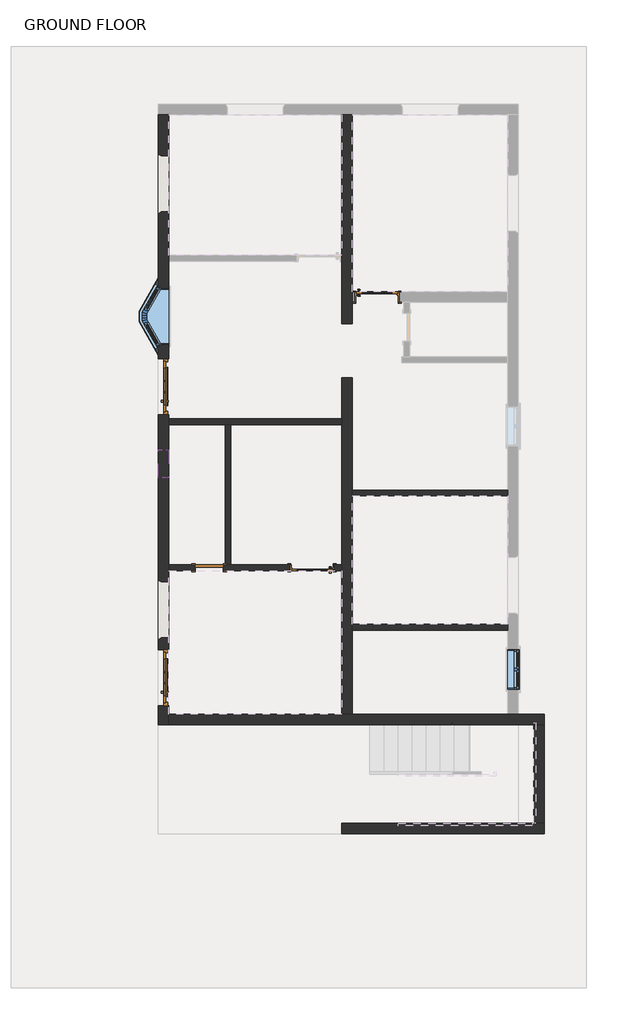
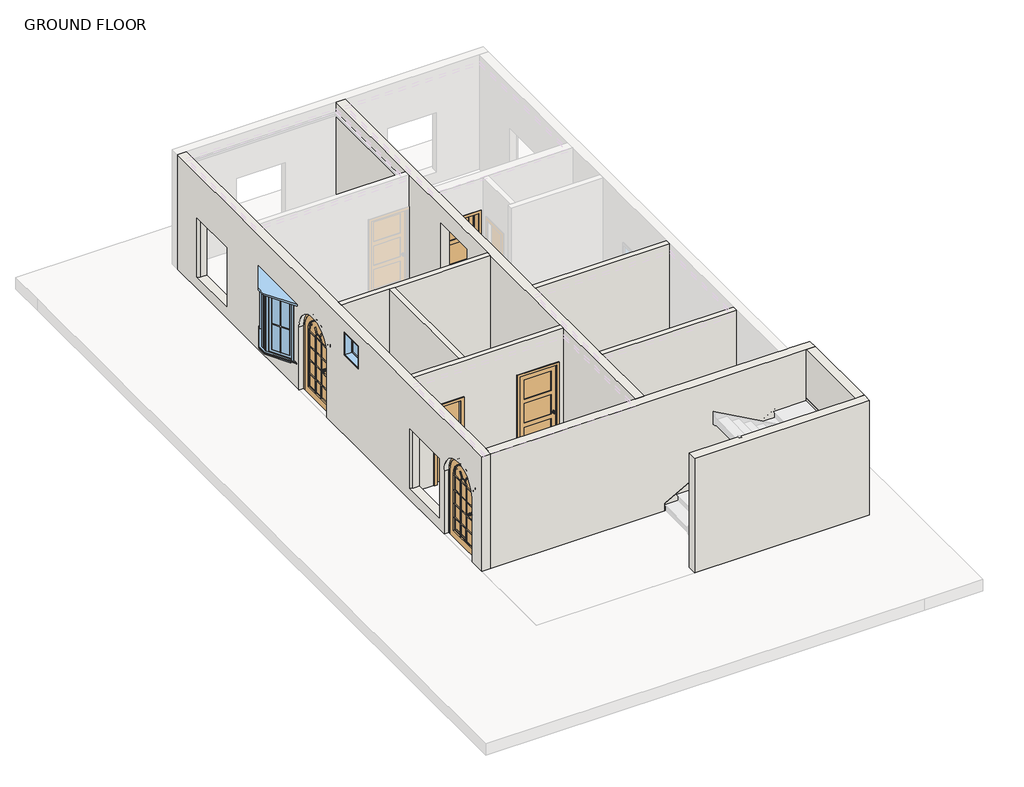
# One storey, part 1 of 2: 10 walls, 5 doors, 3 windows.
"""IFC4 building model written with IfcOpenShell, lengths in millimetres."""

from ifc_helpers import new_model, si_unit, frame, origin, place, context, project, spatial, polyline, circle_curve, outline, extrude, faceted_brep, transform, mapped, element, save
from ifc_brep_helpers import plane_surface, revolved_surface, advanced_brep
from components import door_interior_single_3_panel_vert_wood_interior_door_3_x_7_9905b5e2, door_interior_single_3_panel_vert_wood_interior_door_3_x_7_5540447a, door_arched_single_french_glass_wood_exterior_1219_x_2134mm_67be639c, single_flush_bathroom_flush_door_2_x_7_025d1c86, window_80340324, window_bay_casement_30_degree_angle_30_angle_window_doors_2_b97d1700, window_339605e1

model = new_model("IFC4")

# Units and contexts
model_context = context("Model", 3, world=origin())
ifc_project = project(units=[si_unit("LENGTHUNIT", "METRE", prefix="MILLI")], contexts=[model_context])

# Site, building, storey
site = spatial("IfcSite", under=ifc_project)
building = spatial("IfcBuilding", under=site)
storey = spatial("IfcBuildingStorey", under=building, Name="GROUND FLOOR", Elevation=304.8)

# Doors
placement = place(None, origin())
door_interior_single_3_panel_vert_wood_interior_door_3_x_7_shape = door_interior_single_3_panel_vert_wood_interior_door_3_x_7_9905b5e2(model_context)
element("IfcDoor", 1, ObjectType="Door-Interior-Single-3_Panel_Vert-Wood : 36\" x 84\"", at=placement, inside=storey, context=model_context, shape_type="MappedRepresentation", body=[
    mapped(door_interior_single_3_panel_vert_wood_interior_door_3_x_7_shape, transform((-12603.3436606, 7421.2725873, 304.8), x_axis=(1.0, 0.0, 0.0), y_axis=(0.0, 1.0, 0.0), z_axis=(0.0, 0.0, 1.0))),
])
door_interior_single_3_panel_vert_wood_interior_door_3_x_7_2_shape = door_interior_single_3_panel_vert_wood_interior_door_3_x_7_5540447a(model_context)
element("IfcDoor", 2, ObjectType="Door-Interior-Single-3_Panel_Vert-Wood : INTERIOR DOOR 3' X 7'", at=placement, inside=storey, context=model_context, shape_type="MappedRepresentation", body=[
    mapped(door_interior_single_3_panel_vert_wood_interior_door_3_x_7_2_shape, transform((-14013.0436606, 1534.8225873, 304.8), x_axis=(-1.0, 0.0, 0.0), y_axis=(0.0, -1.0, 0.0), z_axis=(0.0, 0.0, 1.0))),
])
door_arched_single_french_glass_wood_exterior_1219_x_2134mm_shape = door_arched_single_french_glass_wood_exterior_1219_x_2134mm_67be639c(model_context)
element("IfcDoor", 3, ObjectType="Door_Arched_Single_French_Glass_Wood_Exterior : 1219 x 2134mm", at=placement, inside=storey, context=model_context, shape_type="MappedRepresentation", body=[
    mapped(door_arched_single_french_glass_wood_exterior_1219_x_2134mm_shape, transform((-17238.8436606, -849.6024127, 304.8), x_axis=(0.0, 1.0, 0.0), y_axis=(-1.0, 0.0, 0.0), z_axis=(0.0, 0.0, 1.0))),
])
element("IfcDoor", 4, ObjectType="Door_Arched_Single_French_Glass_Wood_Exterior : 1219 x 2134mm", at=placement, inside=storey, context=model_context, shape_type="MappedRepresentation", body=[
    mapped(door_arched_single_french_glass_wood_exterior_1219_x_2134mm_shape, transform((-17238.8436606, 5474.9975873, 304.8), x_axis=(0.0, 1.0, 0.0), y_axis=(-1.0, 0.0, 0.0), z_axis=(0.0, 0.0, 1.0))),
])
single_flush_bathroom_flush_door_2_x_7_shape = single_flush_bathroom_flush_door_2_x_7_025d1c86(model_context)
element("IfcDoor", 5, ObjectType="Single-Flush : BATHROOM FLUSH DOOR 2' X 7'", at=placement, inside=storey, context=model_context, shape_type="MappedRepresentation", body=[
    mapped(single_flush_bathroom_flush_door_2_x_7_shape, transform((-16248.2436606, 1537.9975873, 304.8), x_axis=(1.0, 0.0, 0.0), y_axis=(0.0, 1.0, 0.0), z_axis=(0.0, 0.0, 1.0))),
])

# Walls
element("IfcWall", 6, at=placement, inside=storey, context=model_context, shape_type="AdvancedBrep", body=[
    advanced_brep(
    [(-17353.1436606, -1878.3024127, 3352.8), (-17353.1436606, 11380.4975873, 3352.8), (-17353.1436606, 11380.4975873, 304.8), (-17353.1436606, 6084.5975873, 304.8), (-17353.1436606, 6084.5975873, 1983.4), (-17353.1436606, 4865.3975873, 1983.4), (-17353.1436606, 4865.3975873, 304.8), (-17353.1436606, -240.0024127, 304.8), (-17353.1436606, -240.0024127, 1983.4), (-17353.1436606, -1459.2024127, 1983.4), (-17353.1436606, -1459.2024127, 304.8), (-17353.1436606, -1878.3024127, 304.8), (-17353.1436606, 1268.1225873, 2184.4), (-17353.1436606, -20.9274127, 2184.4), (-17353.1436606, -20.9274127, 609.6), (-17353.1436606, 1268.1225873, 609.6), (-17353.1436606, 3493.7975873, 3048.0), (-17353.1436606, 3493.7975873, 2438.4), (-17353.1436606, 4103.3975873, 2438.4), (-17353.1436606, 4103.3975873, 3048.0), (-17353.1436606, 7643.5225873, 2489.2), (-17353.1436606, 6354.4725873, 2489.2), (-17353.1436606, 6354.4725873, 914.4), (-17353.1436606, 7643.5225873, 914.4), (-17353.1436606, 10526.4225873, 2184.4), (-17353.1436606, 9237.3725873, 2184.4), (-17353.1436606, 9237.3725873, 609.6), (-17353.1436606, 10526.4225873, 609.6), (-17124.5436606, 11380.4975873, 3352.8), (-17124.5436606, 8332.4975873, 3352.8), (-17124.5436606, 8205.4975873, 3352.8), (-17124.5436606, 4776.4975873, 3352.8), (-17124.5436606, 4649.4975873, 3352.8), (-17124.5436606, 1601.4975873, 3352.8), (-17124.5436606, 1474.4975873, 3352.8), (-17124.5436606, -1649.7024127, 3352.8), (-17124.5436606, -1878.3024127, 3352.8), (-17124.5436606, -1878.3024127, 304.8), (-17124.5436606, -1649.7024127, 304.8), (-17124.5436606, -1459.2024127, 304.8), (-17124.5436606, -1459.2024127, 1983.4), (-17124.5436606, -240.0024127, 1983.4), (-17124.5436606, -240.0024127, 304.8), (-17124.5436606, 1474.4975873, 304.8), (-17124.5436606, 1601.4975873, 304.8), (-17124.5436606, 4649.4975873, 304.8), (-17124.5436606, 4776.4975873, 304.8), (-17124.5436606, 4865.3975873, 304.8), (-17124.5436606, 4865.3975873, 1983.4), (-17124.5436606, 6084.5975873, 1983.4), (-17124.5436606, 6084.5975873, 304.8), (-17124.5436606, 8205.4975873, 304.8), (-17124.5436606, 8332.4975873, 304.8), (-17124.5436606, 11380.4975873, 304.8), (-17124.5436606, 13.9975873, 2184.4), (-17124.5436606, 1233.1975873, 2184.4), (-17124.5436606, 1233.1975873, 609.6), (-17124.5436606, 13.9975873, 609.6), (-17124.5436606, 3493.7975873, 2438.4), (-17124.5436606, 3493.7975873, 3048.0), (-17124.5436606, 4103.3975873, 3048.0), (-17124.5436606, 4103.3975873, 2438.4), (-17124.5436606, 6389.3975873, 2489.2), (-17124.5436606, 7608.5975873, 2489.2), (-17124.5436606, 7608.5975873, 914.4), (-17124.5436606, 6389.3975873, 914.4), (-17124.5436606, 9272.2975873, 2184.4), (-17124.5436606, 10491.4975873, 2184.4), (-17124.5436606, 10491.4975873, 609.6), (-17124.5436606, 9272.2975873, 609.6), (-17292.6517862, 13.9975873, 2184.4), (-17292.6517862, 1233.1975873, 2184.4), (-17292.6517862, 13.9975873, 609.6), (-17292.6517862, 1233.1975873, 609.6), (-17292.6517862, 6389.3975873, 2489.2), (-17292.6517862, 7608.5975873, 2489.2), (-17292.6517862, 6389.3975873, 914.4), (-17292.6517862, 7608.5975873, 914.4), (-17292.6517862, 9272.2975873, 2184.4), (-17292.6517862, 10491.4975873, 2184.4), (-17292.6517862, 9272.2975873, 609.6), (-17292.6517862, 10491.4975873, 609.6)],
    [
        (0, 1),
        (1, 2),
        (2, 3),
        (3, 4),
        (4, 5, circle_curve(frame((-17353.1436606, 5474.9975873, 1983.4), z_axis=(1.0, 0.0, 0.0), x_axis=(0.0, 1.0, 0.0)), 609.6)),
        (5, 6),
        (6, 7),
        (7, 8),
        (8, 9, circle_curve(frame((-17353.1436606, -849.6024127, 1983.4), z_axis=(1.0, 0.0, 0.0), x_axis=(0.0, 1.0, 0.0)), 609.6)),
        (9, 10),
        (10, 11),
        (11, 0),
        (12, 13),
        (13, 14),
        (14, 15),
        (15, 12),
        (16, 17),
        (17, 18),
        (18, 19),
        (19, 16),
        (20, 21),
        (21, 22),
        (22, 23),
        (23, 20),
        (24, 25),
        (25, 26),
        (26, 27),
        (27, 24),
        (28, 29),
        (29, 30),
        (30, 31),
        (31, 32),
        (32, 33),
        (33, 34),
        (34, 35),
        (35, 36),
        (36, 37),
        (37, 38),
        (38, 39),
        (39, 40),
        (40, 41, circle_curve(frame((-17124.5436606, -849.6024127, 1983.4), z_axis=(-1.0, 0.0, 0.0), x_axis=(0.0, 1.0, 0.0)), 609.6)),
        (41, 42),
        (42, 43),
        (43, 44),
        (44, 45),
        (45, 46),
        (46, 47),
        (47, 48),
        (48, 49, circle_curve(frame((-17124.5436606, 5474.9975873, 1983.4), z_axis=(-1.0, 0.0, 0.0), x_axis=(0.0, 1.0, 0.0)), 609.6)),
        (49, 50),
        (50, 51),
        (51, 52),
        (52, 53),
        (53, 28),
        (54, 55),
        (55, 56),
        (56, 57),
        (57, 54),
        (58, 59),
        (59, 60),
        (60, 61),
        (61, 58),
        (62, 63),
        (63, 64),
        (64, 65),
        (65, 62),
        (66, 67),
        (67, 68),
        (68, 69),
        (69, 66),
        (2, 53),
        (50, 3),
        (37, 11),
        (10, 39),
        (42, 7),
        (6, 47),
        (0, 36),
        (28, 1),
        (70, 13),
        (12, 71),
        (71, 55),
        (54, 70),
        (72, 57),
        (56, 73),
        (73, 15),
        (14, 72),
        (72, 70),
        (71, 73),
        (8, 41),
        (40, 9),
        (4, 49),
        (48, 5),
        (16, 59),
        (58, 17),
        (61, 18),
        (60, 19),
        (74, 21),
        (20, 75),
        (75, 63),
        (62, 74),
        (76, 65),
        (64, 77),
        (77, 23),
        (22, 76),
        (76, 74),
        (75, 77),
        (78, 25),
        (24, 79),
        (79, 67),
        (66, 78),
        (80, 69),
        (68, 81),
        (81, 27),
        (26, 80),
        (80, 78),
        (79, 81),
    ],
    [
        plane_surface(frame((-17353.1436606, 11380.4975873, 304.8), z_axis=(-1.0, 0.0, 0.0), x_axis=(0.0, -1.0, 0.0))),
        plane_surface(frame((-17124.5436606, 11380.4975873, 304.8), z_axis=(1.0, 0.0, 0.0), x_axis=(0.0, 1.0, 0.0))),
        plane_surface(frame((-17353.1436606, 11494.7975873, 304.8), z_axis=(0.0, 0.0, -1.0), x_axis=(1.0, 0.0, 0.0))),
        plane_surface(frame((-17353.1436606, -1764.0024127, 3352.8), z_axis=(0.0, 0.0, 1.0), x_axis=(1.0, 0.0, 0.0))),
        plane_surface(frame((-17325.7404762, 11380.4975873, 304.8), z_axis=(0.0, 1.0, 0.0), x_axis=(1.0, 0.0, 0.0))),
        plane_surface(frame((-17353.1436606, -1878.3024127, 304.8), z_axis=(0.0, -1.0, 0.0), x_axis=(1.0, 0.0, 0.0))),
        plane_surface(frame((-17292.6517862, 13.9975873, 2184.4), z_axis=(0.0, 0.0, -1.0), x_axis=(1.0, 0.0, 0.0))),
        plane_surface(frame((-17292.6517862, 13.9975873, 609.6), z_axis=(0.0, 0.0, 1.0), x_axis=(-1.0, 0.0, 0.0))),
        plane_surface(frame((-17292.6517862, 13.9975873, 2184.4), z_axis=(0.0, 1.0, 0.0), x_axis=(0.0, 0.0, -1.0))),
        plane_surface(frame((-17124.5436606, 1233.1975873, 2184.4), z_axis=(0.0, -1.0, 0.0), x_axis=(0.0, 0.0, -1.0))),
        plane_surface(frame((-17292.6517862, 1233.1975873, 2184.4), z_axis=(-0.5000000000000007, -0.8660254037844383, 0.0), x_axis=(0.0, 0.0, -1.0))),
        plane_surface(frame((-17353.1436606, -20.9274127, 2184.4), z_axis=(-0.4999999999999979, 0.8660254037844399, 0.0), x_axis=(0.0, 0.0, -1.0))),
        revolved_surface(polyline([(-17124.5436606, -240.00241269999992, 1983.4), (-17353.1436606, -240.00241269999992, 1983.4)]), (-17353.1436606, -849.6024127, 1983.4), (1.0, 0.0, 0.0)),
        plane_surface(frame((-17353.1436606, -1459.2024127, 1983.4), z_axis=(0.0, 1.0, 0.0), x_axis=(1.0, 0.0, 0.0))),
        plane_surface(frame((-17353.1436606, -240.0024127, 304.8), z_axis=(0.0, -1.0, 0.0), x_axis=(1.0, 0.0, 0.0))),
        revolved_surface(polyline([(-17124.5436606, 6084.597587300001, 1983.4), (-17353.1436606, 6084.597587300001, 1983.4)]), (-17353.1436606, 5474.9975873, 1983.4), (1.0, 0.0, 0.0)),
        plane_surface(frame((-17353.1436606, 4865.3975873, 1983.4), z_axis=(0.0, 1.0, 0.0), x_axis=(1.0, 0.0, 0.0))),
        plane_surface(frame((-17353.1436606, 6084.5975873, 304.8), z_axis=(0.0, -1.0, 0.0), x_axis=(1.0, 0.0, 0.0))),
        plane_surface(frame((-17353.1436606, 3493.7975873, 3048.0), z_axis=(0.0, 1.0, 0.0), x_axis=(1.0, 0.0, 0.0))),
        plane_surface(frame((-17353.1436606, 3493.7975873, 2438.4), z_axis=(0.0, 0.0, 1.0), x_axis=(1.0, 0.0, 0.0))),
        plane_surface(frame((-17353.1436606, 4103.3975873, 2438.4), z_axis=(0.0, -1.0, 0.0), x_axis=(1.0, 0.0, 0.0))),
        plane_surface(frame((-17353.1436606, 4103.3975873, 3048.0), z_axis=(0.0, 0.0, -1.0), x_axis=(1.0, 0.0, 0.0))),
        plane_surface(frame((-17292.6517862, 6389.3975873, 2489.2), z_axis=(0.0, 0.0, -1.0), x_axis=(1.0, 0.0, 0.0))),
        plane_surface(frame((-17292.6517862, 6389.3975873, 914.4), z_axis=(0.0, 0.0, 1.0), x_axis=(-1.0, 0.0, 0.0))),
        plane_surface(frame((-17292.6517862, 6389.3975873, 2489.2), z_axis=(0.0, 1.0, 0.0), x_axis=(0.0, 0.0, -1.0))),
        plane_surface(frame((-17124.5436606, 7608.5975873, 2489.2), z_axis=(0.0, -1.0, 0.0), x_axis=(0.0, 0.0, -1.0))),
        plane_surface(frame((-17292.6517862, 7608.5975873, 2489.2), z_axis=(-0.5000000000000007, -0.8660254037844383, 0.0), x_axis=(0.0, 0.0, -1.0))),
        plane_surface(frame((-17353.1436606, 6354.4725873, 2489.2), z_axis=(-0.4999999999999979, 0.8660254037844399, 0.0), x_axis=(0.0, 0.0, -1.0))),
        plane_surface(frame((-17292.6517862, 9272.2975873, 2184.4), z_axis=(0.0, 0.0, -1.0), x_axis=(1.0, 0.0, 0.0))),
        plane_surface(frame((-17292.6517862, 9272.2975873, 609.6), z_axis=(0.0, 0.0, 1.0), x_axis=(-1.0, 0.0, 0.0))),
        plane_surface(frame((-17292.6517862, 9272.2975873, 2184.4), z_axis=(0.0, 1.0, 0.0), x_axis=(0.0, 0.0, -1.0))),
        plane_surface(frame((-17124.5436606, 10491.4975873, 2184.4), z_axis=(0.0, -1.0, 0.0), x_axis=(0.0, 0.0, -1.0))),
        plane_surface(frame((-17292.6517862, 10491.4975873, 2184.4), z_axis=(-0.5000000000000007, -0.8660254037844383, 0.0), x_axis=(0.0, 0.0, -1.0))),
        plane_surface(frame((-17353.1436606, 9237.3725873, 2184.4), z_axis=(-0.4999999999999979, 0.8660254037844399, 0.0), x_axis=(0.0, 0.0, -1.0))),
    ],
    [
        (0, [[1, 2, 3, 4, 5, 6, 7, 8, 9, 10, 11, 12], [13, 14, 15, 16], [17, 18, 19, 20], [21, 22, 23, 24], [25, 26, 27, 28]]),
        (1, [[29, 30, 31, 32, 33, 34, 35, 36, 37, 38, 39, 40, 41, 42, 43, 44, 45, 46, 47, 48, 49, 50, 51, 52, 53, 54], [55, 56, 57, 58], [59, 60, 61, 62], [63, 64, 65, 66], [67, 68, 69, 70]]),
        (2, [[71, -53, -52, -51, 72, -3]]),
        (2, [[73, -11, 74, -39, -38]]),
        (2, [[75, -7, 76, -47, -46, -45, -44, -43]]),
        (3, [[-1, 77, -36, -35, -34, -33, -32, -31, -30, -29, 78]]),
        (4, [[-2, -78, -54, -71]]),
        (5, [[-12, -73, -37, -77]]),
        (6, [[79, -13, 80, 81, -55, 82]]),
        (7, [[83, -57, 84, 85, -15, 86]]),
        (8, [[-82, -58, -83, 87]]),
        (9, [[-81, 88, -84, -56]]),
        (10, [[-80, -16, -85, -88]]),
        (11, [[-79, -87, -86, -14]]),
        (12, [[-9, 89, -41, 90]]),
        (13, [[-10, -90, -40, -74]]),
        (14, [[-8, -75, -42, -89]]),
        (15, [[-5, 91, -49, 92]]),
        (16, [[-6, -92, -48, -76]]),
        (17, [[-4, -72, -50, -91]]),
        (18, [[-17, 93, -59, 94]]),
        (19, [[-18, -94, -62, 95]]),
        (20, [[-19, -95, -61, 96]]),
        (21, [[-20, -96, -60, -93]]),
        (22, [[97, -21, 98, 99, -63, 100]]),
        (23, [[101, -65, 102, 103, -23, 104]]),
        (24, [[-100, -66, -101, 105]]),
        (25, [[-99, 106, -102, -64]]),
        (26, [[-98, -24, -103, -106]]),
        (27, [[-97, -105, -104, -22]]),
        (28, [[107, -25, 108, 109, -67, 110]]),
        (29, [[111, -69, 112, 113, -27, 114]]),
        (30, [[-110, -70, -111, 115]]),
        (31, [[-109, 116, -112, -68]]),
        (32, [[-108, -28, -113, -116]]),
        (33, [[-107, -115, -114, -26]]),
    ],
),
])
element("IfcWall", 7, at=placement, inside=storey, context=model_context, shape_type="Brep", body=[
    faceted_brep([(-17124.5436606, -1878.3024127, 304.8), (-9199.7436606, -1878.3024127, 304.8), (-8971.1436606, -1878.3024127, 304.8), (-8971.1436606, -1878.3024127, 3352.8), (-9199.7436606, -1878.3024127, 3352.8), (-17124.5436606, -1878.3024127, 3352.8), (-17124.5436606, -1649.7024127, 304.8), (-17124.5436606, -1649.7024127, 3352.8), (-13365.3436606, -1649.7024127, 3352.8), (-13136.7436606, -1649.7024127, 3352.8), (-9758.5436606, -1649.7024127, 3352.8), (-9529.9436606, -1649.7024127, 3352.8), (-8971.1436606, -1649.7024127, 3352.8), (-8971.1436606, -1649.7024127, 304.8), (-9529.9436606, -1649.7024127, 304.8), (-9758.5436606, -1649.7024127, 304.8), (-13136.7436606, -1649.7024127, 304.8), (-13365.3436606, -1649.7024127, 304.8)], [[[0, 1, 2, 3, 4, 5]], [[6, 7, 8, 9, 10, 11, 12, 13, 14, 15, 16, 17]], [[2, 1, 0, 6, 17, 16, 15, 14, 13]], [[5, 4, 3, 12, 11, 10, 9, 8, 7]], [[0, 5, 7, 6]], [[3, 2, 13, 12]]]),
])
element("IfcWall", 8, at=placement, inside=storey, context=model_context, shape_type="Brep", body=[
    faceted_brep([(-13365.3436606, -1649.7024127, 304.8), (-13365.3436606, -1649.7024127, 3352.8), (-13365.3436606, 1474.4975873, 3352.8), (-13365.3436606, 1601.4975873, 3352.8), (-13365.3436606, 4649.4975873, 3352.8), (-13365.3436606, 4776.4975873, 3352.8), (-13365.3436606, 8205.4975873, 3352.8), (-13365.3436606, 8332.4975873, 3352.8), (-13365.3436606, 11380.4975873, 3352.8), (-13365.3436606, 11380.4975873, 304.8), (-13365.3436606, 8332.4975873, 304.8), (-13365.3436606, 8205.4975873, 304.8), (-13365.3436606, 6840.0734188, 304.8), (-13365.3436606, 6840.0734188, 2912.3433381), (-13365.3436606, 5663.8725029, 2912.3433381), (-13365.3436606, 5663.8725029, 304.8), (-13365.3436606, 4776.4975873, 304.8), (-13365.3436606, 4649.4975873, 304.8), (-13365.3436606, 1601.4975873, 304.8), (-13365.3436606, 1474.4975873, 304.8), (-13136.7436606, -1649.7024127, 3352.8), (-13136.7436606, -1649.7024127, 304.8), (-13136.7436606, 179.0975873, 304.8), (-13136.7436606, 306.0975873, 304.8), (-13136.7436606, 3100.0975873, 304.8), (-13136.7436606, 3227.0975873, 304.8), (-13136.7436606, 5663.8725029, 304.8), (-13136.7436606, 5663.8725029, 2912.3433381), (-13136.7436606, 6840.0734188, 2912.3433381), (-13136.7436606, 6840.0734188, 304.8), (-13136.7436606, 7303.7975873, 304.8), (-13136.7436606, 7532.3975873, 304.8), (-13136.7436606, 11380.4975873, 304.8), (-13136.7436606, 11380.4975873, 3352.8), (-13136.7436606, 7532.3975873, 3352.8), (-13136.7436606, 7303.7975873, 3352.8), (-13136.7436606, 3227.0975873, 3352.8), (-13136.7436606, 3100.0975873, 3352.8), (-13136.7436606, 306.0975873, 3352.8), (-13136.7436606, 179.0975873, 3352.8)], [[[0, 1, 2, 3, 4, 5, 6, 7, 8, 9, 10, 11, 12, 13, 14, 15, 16, 17, 18, 19]], [[20, 21, 22, 23, 24, 25, 26, 27, 28, 29, 30, 31, 32, 33, 34, 35, 36, 37, 38, 39]], [[9, 8, 33, 32]], [[1, 0, 21, 20]], [[13, 28, 27, 14]], [[28, 13, 12, 29]], [[14, 27, 26, 15]], [[9, 32, 31, 30, 29, 12, 11, 10]], [[21, 0, 19, 18, 17, 16, 15, 26, 25, 24, 23, 22]], [[8, 7, 6, 5, 4, 3, 2, 1, 20, 39, 38, 37, 36, 35, 34, 33]]]),
])
element("IfcWall", 9, at=placement, inside=storey, context=model_context, shape_type="Brep", body=[
    faceted_brep([(-13365.3436606, -4240.5024127, 304.8), (-8971.1436606, -4240.5024127, 304.8), (-8971.1436606, -4240.5024127, 3352.8), (-13365.3436606, -4240.5024127, 3352.8), (-13365.3436606, -4011.9024127, 304.8), (-13365.3436606, -4011.9024127, 3352.8), (-9199.7436606, -4011.9024127, 3352.8), (-8971.1436606, -4011.9024127, 3352.8), (-8971.1436606, -4011.9024127, 304.8), (-9199.7436606, -4011.9024127, 304.8)], [[[0, 1, 2, 3]], [[4, 5, 6, 7, 8, 9]], [[1, 0, 4, 9, 8]], [[3, 2, 7, 6, 5]], [[0, 3, 5, 4]], [[2, 1, 8, 7]]]),
])
element("IfcWall", 10, at=placement, inside=storey, context=model_context, shape_type="SweptSolid", body=[
    extrude(outline(polyline([(-8971.1436606, -1878.3024127), (-8971.1436606, -4011.9024127), (-9199.7436606, -4011.9024127), (-9199.7436606, -1878.3024127), (-8971.1436606, -1878.3024127)])), frame((0.0, 0.0, 304.8), z_axis=(0.0, 0.0, 1.0), x_axis=(1.0, 0.0, 0.0)), (0.0, 0.0, 1.0), 3048.0),
])
element("IfcWall", 11, ObjectType="INNER WALL 5\"", at=placement, inside=storey, context=model_context, shape_type="Brep", body=[
    faceted_brep([(-17124.5436606, 4649.4975873, 304.8), (-15905.3436606, 4649.4975873, 304.8), (-15778.3436606, 4649.4975873, 304.8), (-13365.3436606, 4649.4975873, 304.8), (-13365.3436606, 4649.4975873, 3352.8), (-15778.3436606, 4649.4975873, 3352.8), (-15905.3436606, 4649.4975873, 3352.8), (-17124.5436606, 4649.4975873, 3352.8), (-17124.5436606, 4776.4975873, 304.8), (-17124.5436606, 4776.4975873, 3352.8), (-13365.3436606, 4776.4975873, 3352.8), (-13365.3436606, 4776.4975873, 304.8)], [[[0, 1, 2, 3, 4, 5, 6, 7]], [[8, 9, 10, 11]], [[3, 2, 1, 0, 8, 11]], [[7, 6, 5, 4, 10, 9]], [[0, 7, 9, 8]], [[4, 3, 11, 10]]]),
])
element("IfcWall", 12, ObjectType="INNER WALL 5\"", at=placement, inside=storey, context=model_context, shape_type="Brep", body=[
    faceted_brep([(-15943.4436606, 1474.4975873, 2336.8), (-15943.4436606, 1474.4975873, 304.8), (-14495.6436606, 1474.4975873, 304.8), (-14495.6436606, 1474.4975873, 2463.8), (-13530.4436606, 1474.4975873, 2463.8), (-13530.4436606, 1474.4975873, 304.8), (-13365.3436606, 1474.4975873, 304.8), (-13365.3436606, 1474.4975873, 3352.8), (-17124.5436606, 1474.4975873, 3352.8), (-17124.5436606, 1474.4975873, 304.8), (-16553.0436606, 1474.4975873, 304.8), (-16553.0436606, 1474.4975873, 2336.8), (-14495.6436606, 1601.4975873, 304.8), (-15778.3436606, 1601.4975873, 304.8), (-15905.3436606, 1601.4975873, 304.8), (-15943.4436606, 1601.4975873, 304.8), (-15943.4436606, 1601.4975873, 2336.8), (-16553.0436606, 1601.4975873, 2336.8), (-16553.0436606, 1601.4975873, 304.8), (-17124.5436606, 1601.4975873, 304.8), (-17124.5436606, 1601.4975873, 3352.8), (-15905.3436606, 1601.4975873, 3352.8), (-15778.3436606, 1601.4975873, 3352.8), (-13365.3436606, 1601.4975873, 3352.8), (-13365.3436606, 1601.4975873, 304.8), (-13530.4436606, 1601.4975873, 304.8), (-13530.4436606, 1601.4975873, 2463.8), (-14495.6436606, 1601.4975873, 2463.8)], [[[0, 1, 2, 3, 4, 5, 6, 7, 8, 9, 10, 11]], [[12, 13, 14, 15, 16, 17, 18, 19, 20, 21, 22, 23, 24, 25, 26, 27]], [[24, 6, 5, 25]], [[10, 9, 19, 18]], [[2, 1, 15, 14, 13, 12]], [[8, 7, 23, 22, 21, 20]], [[9, 8, 20, 19]], [[7, 6, 24, 23]], [[27, 3, 2, 12]], [[3, 27, 26, 4]], [[4, 26, 25, 5]], [[16, 15, 1, 0]], [[17, 16, 0, 11]], [[18, 17, 11, 10]]]),
])
element("IfcWall", 13, ObjectType="INNER WALL 5\"", at=placement, inside=storey, context=model_context, shape_type="SweptSolid", body=[
    extrude(outline(polyline([(-15778.3436606, 4649.4975873), (-15778.3436606, 1601.4975873), (-15905.3436606, 1601.4975873), (-15905.3436606, 4649.4975873), (-15778.3436606, 4649.4975873)])), frame((0.0, 0.0, 304.8), z_axis=(0.0, 0.0, 1.0), x_axis=(1.0, 0.0, 0.0)), (0.0, 0.0, 1.0), 3048.0),
])
element("IfcWall", 14, ObjectType="INNER WALL 5\"", at=placement, inside=storey, context=model_context, shape_type="SweptSolid", body=[
    extrude(outline(polyline([(-13136.7436606, 306.0975873), (-9758.5436606, 306.0975873), (-9758.5436606, 179.0975873), (-13136.7436606, 179.0975873), (-13136.7436606, 306.0975873)])), frame((0.0, 0.0, 304.8), z_axis=(0.0, 0.0, 1.0), x_axis=(1.0, 0.0, 0.0)), (0.0, 0.0, 1.0), 3048.0),
])
element("IfcWall", 15, ObjectType="INNER WALL 5\"", at=placement, inside=storey, context=model_context, shape_type="SweptSolid", body=[
    extrude(outline(polyline([(-9758.5436606, 3100.0975873), (-13136.7436606, 3100.0975873), (-13136.7436606, 3227.0975873), (-9758.5436606, 3227.0975873), (-9758.5436606, 3100.0975873)])), frame((0.0, 0.0, 304.8), z_axis=(0.0, 0.0, 1.0), x_axis=(1.0, 0.0, 0.0)), (0.0, 0.0, 1.0), 3048.0),
])

# Windows
window_shape = window_80340324(model_context)
element("IfcWindow", 16, ObjectType="Fixed : 24\" x 24\"", at=placement, inside=storey, context=model_context, shape_type="MappedRepresentation", body=[
    mapped(window_shape, transform((-17238.8436606, 3760.4975873, 1524.0), x_axis=(0.0, -1.0, 0.0), y_axis=(1.0, 0.0, 0.0), z_axis=(0.0, 0.0, 1.0))),
])
window_bay_casement_30_degree_angle_30_angle_window_doors_2_shape = window_bay_casement_30_degree_angle_30_angle_window_doors_2_b97d1700(model_context)
element("IfcWindow", 17, ObjectType="Window-Bay-Casement-30_Degree_Angle : 30 ANGLE WINDOW DOORS 2", at=placement, inside=storey, context=model_context, shape_type="MappedRepresentation", body=[
    mapped(window_bay_casement_30_degree_angle_30_angle_window_doors_2_shape, transform((-17238.8436606, 6998.9975873, 304.8), x_axis=(0.0, 1.0, 0.0), y_axis=(-1.0, 0.0, 0.0), z_axis=(0.0, 0.0, 1.0))),
])
window_2_shape = window_339605e1(model_context)
element("IfcWindow", 18, ObjectType="Window-Casement-Double : 34\" x 36\"", at=placement, inside=storey, context=model_context, shape_type="MappedRepresentation", body=[
    mapped(window_2_shape, transform((-9644.2436606, -671.8024127, 304.8), x_axis=(0.0, -1.0, 0.0), y_axis=(1.0, 0.0, 0.0), z_axis=(0.0, 0.0, 1.0))),
])

save(model, "model.ifc")

# Revit data of these elements
# Type "Door-Interior-Single-3_Panel_Vert-Wood : 36\" x 84\""
#   Type Mark = "9"
#   Assembly Code = "C1020300"
#   Analytic Construction = "Wooden"
#   Top Rail = 0' - 4 11/16"
#   Thickness = 0' - 1 3/8"
#   Thermal Resistance (R) = 2.5876 (h·ft²·°F)/BTU
#   Swing Angle [instance default] = 90.00°
#   Stiles = 0' - 4 3/4"
#   Rough Width = 3' - 2"
#   Rough Height = 7' - 1"
#   Intermediate Rail = 0' - 4 1/2"
#   Height = 7' - 0"
#   Width = 3' - 0"
#   Heat Transfer Coefficient (U) = 0.3865 BTU/(h·ft²·°F)
#   Bottom Rail = 0' - 9 1/8"
#   Trim Material = Cherry
#   Panel Material = Cherry
#   Frame Material = Cherry
#   Door Handle Material = Aluminum
#   Visual Light Transmittance = 0
#   Solar Heat Gain Coefficient = 0
#   Wall Closure = (empty or 0)
#   Function = (empty or 0)
# Type "Door-Interior-Single-3_Panel_Vert-Wood : INTERIOR DOOR 3' X 7'"
#   Type Mark = "10"
#   Assembly Code = "C1020300"
#   Analytic Construction = "Wooden"
#   Top Rail = 0' - 4 11/16"
#   Thickness = 0' - 1 3/8"
#   Thermal Resistance (R) = 2.5876 (h·ft²·°F)/BTU
#   Swing Angle [instance default] = 90.00°
#   Stiles = 0' - 4 3/4"
#   Rough Width = 3' - 2"
#   Rough Height = 7' - 1"
#   Intermediate Rail = 0' - 4 1/2"
#   Height = 7' - 0"
#   Width = 3' - 0"
#   Heat Transfer Coefficient (U) = 0.3865 BTU/(h·ft²·°F)
#   Bottom Rail = 0' - 9 1/8"
#   Trim Material = Cherry
#   Panel Material = Cherry
#   Frame Material = Cherry
#   Door Handle Material = Aluminum
#   Visual Light Transmittance = 0
#   Solar Heat Gain Coefficient = 0
#   Wall Closure = (empty or 0)
#   Function = (empty or 0)
# Type "Door_Arched_Single_French_Glass_Wood_Exterior : 1219 x 2134mm"
#   Type Mark = "12"
#   Type Comments = "External Single"
#   Operation = "SingleSwingRight"
#   Keynote = "L20"
#   Analytic Construction = "<None>"
#   Wrap Layers (Int) from Ext = 0' - 6.98819"
#   Wrap Layers (Ext) from Ext = 0' - 4.03543"
#   Thickness = 0' - 1.73228"
#   Stile Shutting = 0' - 5.90551"
#   Stile - Top Rail = 0' - 5.90551"
#   Stile - Hanging = 0' - 5.90551"
#   Stile - Bottom Rail = 0' - 6.88976"
#   Rough Width = 4' - 0"
#   Rough Height = 7' - 0"
#   O/A Frame Width = 0' - 2.51969"
#   Handle Z Distance = 3' - 5.33858"
#   Glazing Thickness = 0' - 0.94488"
#   Glazing Bar Thickness = 0' - 0.7874"
#   FrameWidth = 0' - 1.65354"
#   FrameOffset - External = 0' - 0.98425"
#   FrameDepth = 0' - 3.50394"
#   Door Panel Width = 3' - 7.94488"
#   Handle X Distance = 0' - 2.95276"
#   Height = 7' - 0"
#   Structural Tolerance = 0' - 0.25591"
#   Tolerance = 0' - 0.11811"
#   Undercut = 0' - 0.15748"
#   Width = 4' - 0"
#   Door Panel Thickness = 0' - 1.73228"
#   Door Panel Height = 6' - 9.81496"
#   Cavity Closer Width = 0' - 1.9685"
#   Cavity Closer Offset from Ext = 0' - 4.03543"
#   Cavity Closer Depth = 0' - 3.34646"
#   Vis - Ironmongery = yes
#   Vis - Cavity Closers = yes
#   Define Thermal Properties by = 1
#   Material Glass = Door - Glazing
#   Handle Style = element 451349
#   Material Door = Door - Panel
#   Material Frame = BROWN
#   Material Ironmongery = Door - Handle
#   Function = (empty or 0)
#   Wall Closure = (empty or 0)
#   Assembly Code = ""
# Type "Single-Flush : BATHROOM FLUSH DOOR 2' X 7'"
#   Type Mark = "8"
#   Construction Type Id = "MDOOR"
#   Assembly Code = "C1020"
#   Analytic Construction = "Metal"
#   Thickness = 0' - 2"
#   Heat Transfer Coefficient (U) = 0.651978 BTU/(h·ft²·°F)
#   Height = 6' - 8"
#   Trim Projection Ext = 0' - 1"
#   Trim Projection Int = 0' - 1"
#   Trim Width = 0' - 3"
#   Width = 2' - 0"
#   Define Thermal Properties by = 1
#   Door Material = Door - Panel
#   Frame Material = Door - Frame
#   Visual Light Transmittance = 0
#   Solar Heat Gain Coefficient = 0
#   Function = (empty or 0)
#   Wall Closure = (empty or 0)
# Type
#   Assembly Code = "B2010"
#   Layers, outside or top first: 0' - 9" "TERRACOTTA" (function 1)
# Type "INNER WALL 5\""
#   Assembly Code = "B2010"
#   Layers, outside or top first: 0' - 5" "TERRACOTTA" (function 1)
# Type "Fixed : 24\" x 24\""
#   Type Mark = "3"
#   Construction Type Id = "GSP4R"
#   Assembly Code = "B2020100"
#   Analytic Construction = "1/8 in Pilkington single glazing"
#   Visual Light Transmittance = 0.9
#   Solar Heat Gain Coefficient = 0.78
#   Heat Transfer Coefficient (U) = 0.6496 BTU/(h·ft²·°F)
#   Height = 2' - 0"
#   Default Sill Height = 3' - 0"
#   Width = 2' - 0"
#   Window Inset = 0' - 0 3/4"
#   Define Thermal Properties by = 1
#   Define Thermal Properties by = 1
#   Glass Pane Material = Glass
#   Sash Material = Sash
#   Wall Closure = (empty or 0)
# Type "Window-Bay-Casement-30_Degree_Angle : 30 ANGLE WINDOW DOORS 2"
#   Type Mark = "20"
#   Fire Rating = "0.5h"
#   Assembly Code = "B2020100"
#   Analytic Construction = "Double glazing - domestic"
#   Width of Middle Sash = 0' - 2.5827"
#   Width = 4' - 0"
#   Visual Light Transmittance = 0.81
#   Thermal Resistance (R) = 1.8146 (h·ft²·°F)/BTU
#   Solar Heat Gain Coefficient = 0.76
#   Rough Width = 4' - 0 1/2"
#   Rough Height = 5' - 0 1/2"
#   Length 2 = 0' - 7.25458"
#   Length 1 = 1' - 8.70865"
#   Wall Thickness [instance default] = 0' - 6"
#   Trim Width = 4' - 4 43/64"
#   Trim Height = 5' - 0"
#   Height 1 = 5' - 2"
#   Height = 5' - 0"
#   Heat Transfer Coefficient (U) = 0.5511 BTU/(h·ft²·°F)
#   Depth = 1' - 2"
#   Default Sill Height = 2' - 0"
#   Angle = 30.00°
#   Muntin Visibility = yes
#   Interior Trim Visibility [instance default] = yes
#   Exterior Trim Visibility [instance default] = yes
#   Muntin Pattern = Muntin Pattern_2x2 : Muntin Pattern_2x2
#   Interior Trim Material = Wood - Stained
#   Exterior Trim Material = Clad - White
#   Exterior Trim = element 398720
#   Interior Trim = Trim-Window-Interior-Flat : Picture Frame
#   Interior Frame Material = Wood - Stained
#   Glass Panel Material = Glass
#   Exterior Frame Material = Clad - White
#   Wall Closure = (empty or 0)
# Type "Window-Casement-Double : 34\" x 36\""
#   Type Mark = "14"
#   Fire Rating = "0.5h"
#   Assembly Code = "B2020100"
#   Analytic Construction = "Double glazing - domestic"
#   Frame Extension [instance default] = 0' - 0 1/4"
#   Window Inset [instance default] = 0' - 0"
#   Wall Thickness [instance default] = 0' - 6"
#   Interior Wall Closure [instance default] = 0' - 2 1/4"
#   Half Width = 1' - 5"
#   Visual Light Transmittance = 0.81
#   Thermal Resistance (R) = 1.8146 (h·ft²·°F)/BTU
#   Solar Heat Gain Coefficient = 0.76
#   Rough Width = 2' - 10 1/2"
#   Rough Height = 3' - 0 1/2"
#   Height = 3' - 0"
#   Heat Transfer Coefficient (U) = 0.5511 BTU/(h·ft²·°F)
#   Exterior Wall Closure [instance default] = 0' - 1 1/4"
#   Extension Jamb [instance default] = 0' - 2 1/4"
#   Default Sill Height = 3' - 0"
#   Width = 2' - 10"
#   Define Thermal Properties by = 0
#   Muntin Visibility = yes
#   Interior Trim Visibility [instance default] = yes
#   Exterior Trim Visibility [instance default] = yes
#   Extension Jamb Visibility [instance default] = yes
#   Interior Trim Material = Wood - Stained
#   Muntin Pattern = Muntin Pattern_2x2 : Muntin Pattern_2x2
#   Interior Trim = Trim-Window-Interior-Flat : Picture Frame
#   Interior Frame Material = Wood - Stained
#   Glass Panel Material = Glass
#   Exterior Trim Material = Clad - White
#   Exterior Trim = Trim-Window-Exterior-Flat : with Sill
#   Exterior Frame Material = Clad - White
#   Wall Closure = (empty or 0)
# Element 1 (IfcDoor, "Door-Interior-Single-3_Panel_Vert-Wood : 36\" x 84\"")
#   Swing Angle = 90.00°
#   Phase Created = New Construction
#   Materials on its faces: "Cherry", "Aluminum"
# Element 2 (IfcDoor, "Door-Interior-Single-3_Panel_Vert-Wood : INTERIOR DOOR 3' X 7'")
#   Phase Created = New Construction
#   Materials on its faces: "Cherry", "Aluminum"
# Elements 3, 4 (IfcDoor, "Door_Arched_Single_French_Glass_Wood_Exterior : 1219 x 2134mm")
#   Phase Created = New Construction
#   Materials on its faces: "Door - Panel", "Door - Handle", "BROWN", "Door - Glazing"
# Element 5 (IfcDoor, "Single-Flush : BATHROOM FLUSH DOOR 2' X 7'")
#   Phase Created = New Construction
#   Materials on its faces: "Door - Frame", "Door - Panel"
# Elements 6, 7, 8, 9, 10 (IfcWall)
#   Top Offset = 0' - 0"
#   Base Offset = 0' - 0"
#   wall height = 10' - 0"
#   Phase Created = New Construction
#   Base Constraint = GROUND FLOOR
#   Top Constraint = FIRST FLOOR
#   Materials on its faces: "TERRACOTTA"
# Elements 11, 12, 13, 14, 15 (IfcWall, "INNER WALL 5\"")
#   Top Offset = 0' - 0"
#   Base Offset = 0' - 0"
#   wall height = 10' - 0"
#   Phase Created = New Construction
#   Base Constraint = GROUND FLOOR
#   Top Constraint = FIRST FLOOR
#   Materials on its faces: "TERRACOTTA"
# Element 16 (IfcWindow, "Fixed : 24\" x 24\"")
#   Mark = "10"
#   Phase Created = New Construction
#   Materials on its faces: "Sash", "Glass"
# Element 17 (IfcWindow, "Window-Bay-Casement-30_Degree_Angle : 30 ANGLE WINDOW DOORS 2")
#   Mark = "1"
#   Interior Trim Visibility = yes
#   Exterior Trim Visibility = yes
#   Phase Created = New Construction
#   Materials on its faces: "Clad - White", "Wood - Stained", "Glass"
# Element 18 (IfcWindow, "Window-Casement-Double : 34\" x 36\"")
#   Mark = "8"
#   Window Inset = 0' - 0"
#   Interior Wall Closure = 0' - 2 1/4"
#   Frame Extension = 0' - 0 1/4"
#   Exterior Wall Closure = 0' - 1 1/4"
#   Interior Trim Visibility = yes
#   Exterior Trim Visibility = yes
#   Phase Created = New Construction
#   Materials on its faces: "Wood - Stained", "Glass", "Clad - White"
# Materials
#   "Cherry": class "Wood", colour RGB 226 177 128, transparency 0, Description = "Prunus Serotina", Cost = 0
#   "Aluminum": class "Metal", colour RGB 247 247 247, transparency 0, Description = "Aluminum 6061", Cost = 0
#   "Door - Glazing": colour RGB 218 227 224, transparency 0.85
#   "Door - Panel": class "Wood", colour RGB 210 159 95, transparency 0, Cost = 0
#   "BROWN": class "Generic", colour RGB 120 120 120, transparency 0, Cost = 0
#   "Door - Handle": colour RGB 0 0 0, transparency 0, Keynote = "P21"
#   "Door - Frame": colour RGB 118 70 51, transparency 0, Cost = 0
#   "TERRACOTTA": class "Generic", colour RGB 190 112 66, transparency 0, Cost = 0
#   "Glass": class "Glass", colour RGB 0 128 192, transparency 0.75, Description = "Soda Lime Glass", Cost = 0
#   "Sash": class "Wood", colour RGB 224 178 126, transparency 0, Cost = 0
#   "Wood - Stained": class "Wood", colour RGB 224 178 126, transparency 0, Cost = 0
#   "Clad - White": class "Wood", colour RGB 30 30 30, transparency 0, Cost = 0
